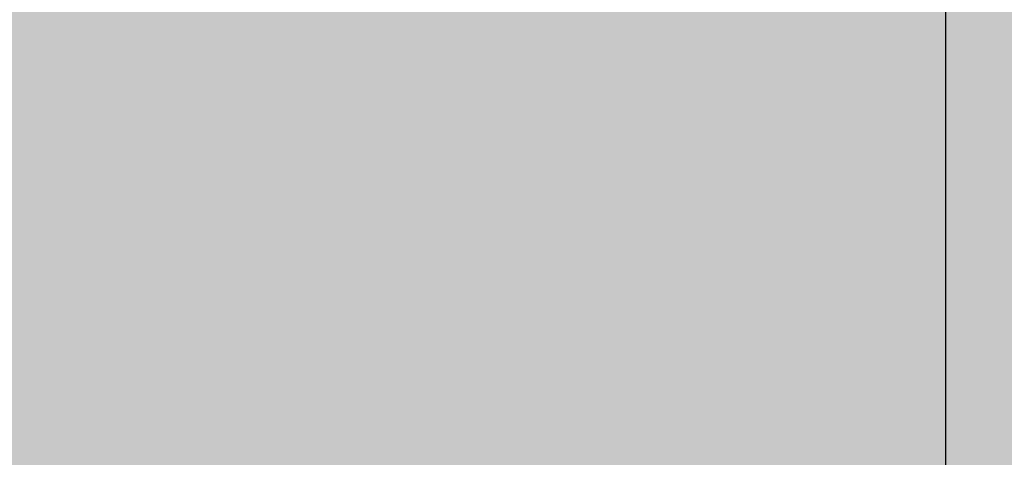
# Model space of a CAD drawing. Units: millimetres. Extents: x 0 to 2267, y 0 to 1823.
# Tile 148 of 256: x 1833.61 to 1844.05, y 1112.67 to 1117.32. Entities that reach past the tile are written whole.
import ezdxf

# ---------------------------------------------------------------- set-up
doc = ezdxf.new("R2010")
doc.units = ezdxf.units.MM
doc.header["$MEASUREMENT"] = 0
doc.layers.add('M-DIMS', color=2, linetype='Continuous', lineweight=25)
doc.layers.add('M-HATC', color=252, linetype='Continuous', lineweight=18)
doc.styles.get("Standard").update_dxf_attribs({"font": 'arial.ttf'})
doc.dimstyles.get("Standard").update_dxf_attribs({"dimtxt": 7, "dimasz": 4, "dimexe": 0.18, "dimexo": 0.0625, "dimgap": 0.09, "dimtad": 0, "dimdec": 0, "dimzin": 0, "dimdsep": 46, "dimtxsty": 'Standard', "dimcen": 0.09, "dimadec": 0, "dimazin": 0, "dimtfac": 1, "dimtdec": 0, "dimtofl": 0, "dimtmove": 0, "dimatfit": 3, "dimfxl": 1, "dimtolj": 1, "dimtzin": 0, "dimarcsym": 0})

# ---------------------------------------------------------------- blocks, each defined once
blk = doc.blocks.new('*D1')
at = {"layer": 'Defpoints', "color": 0, "transparency": 16777216}
for p in [(1593.429, 1127.417), (1843.429, 1127.417), (1843.429, 955.628)]:
    blk.add_point(p, dxfattribs=at)
at = {"layer": 'M-DIMS', "color": 0, "lineweight": -2, "transparency": 16777216}
for p, q in [((1593.429, 1127.355), (1593.429, 955.448)), ((1843.429, 1127.355), (1843.429, 955.448)), ((1597.429, 955.628), (1710.558, 955.628)), ((1839.429, 955.628), (1726.3, 955.628))]:
    blk.add_line(p, q, dxfattribs=at)
at = {"layer": 'M-DIMS', "color": 0, "transparency": 16777216}
for points in [[(1597.429, 956.294), (1597.429, 954.961), (1593.429, 955.628)], [(1839.429, 956.294), (1839.429, 954.961), (1843.429, 955.628)]]:
    blk.add_solid(points, dxfattribs=at)
at = {"layer": 'M-DIMS', "color": 0, "transparency": 16777216, "insert": (1718.429, 955.628), "char_height": 7, "attachment_point": 5}
blk.add_mtext('\\A1;250', dxfattribs=at)

msp = doc.modelspace()

# ---------------------------------------------------------------- hatches: boundary and pattern name
at = {"layer": 'M-HATC'}
h = msp.add_hatch(color=256, dxfattribs=at)
h.dxf.hatch_style = 1
h.paths.add_polyline_path([(2065.771, 1618.062, 0.236068), (2055.771, 1638.062), (1381.087, 1638.062, 0.236068), (1371.087, 1618.062), (1371.087, 1603.062), (2055.771, 1603.062), (2065.771, 1603.062)])
h.paths.add_polyline_path([(2062.772, 1550.296), (2062.772, 1560.296), (1374.086, 1560.296), (1374.086, 1550.296), (1374.086, 1540.296), (1384.086, 1540.296), (1389.086, 1540.296), (2062.772, 1540.296)])
h.paths.add_polyline_path([(1930.929, 1282.766), (1505.929, 1282.766), (1587.628, 1235.597, 0.131652), (1600.128, 1232.247), (1836.73, 1232.247, 0.131652), (1849.23, 1235.597)])
h.paths.add_polyline_path([(1930.929, 1117.417), (1905.929, 1117.417), (1505.929, 1117.417), (1505.929, 1077.417), (1930.929, 1077.417)])

# ---------------------------------------------------------------- dimensions: what is measured, and where the dimension line sits
at = {"layer": 'M-DIMS'}
dim = msp.add_linear_dim(base=(1843.429, 955.628), p1=(1593.429, 1127.417), p2=(1843.429, 1127.417), dimstyle='Standard', override={"dimclrd": 0, "dimclre": 0, "dimclrt": 0}, dxfattribs=at)
dim.commit()
dim.dimension.update_dxf_attribs({"geometry": '*D1', "text_midpoint": (1718.429, 955.628)})

doc.saveas('drawing.dxf')
